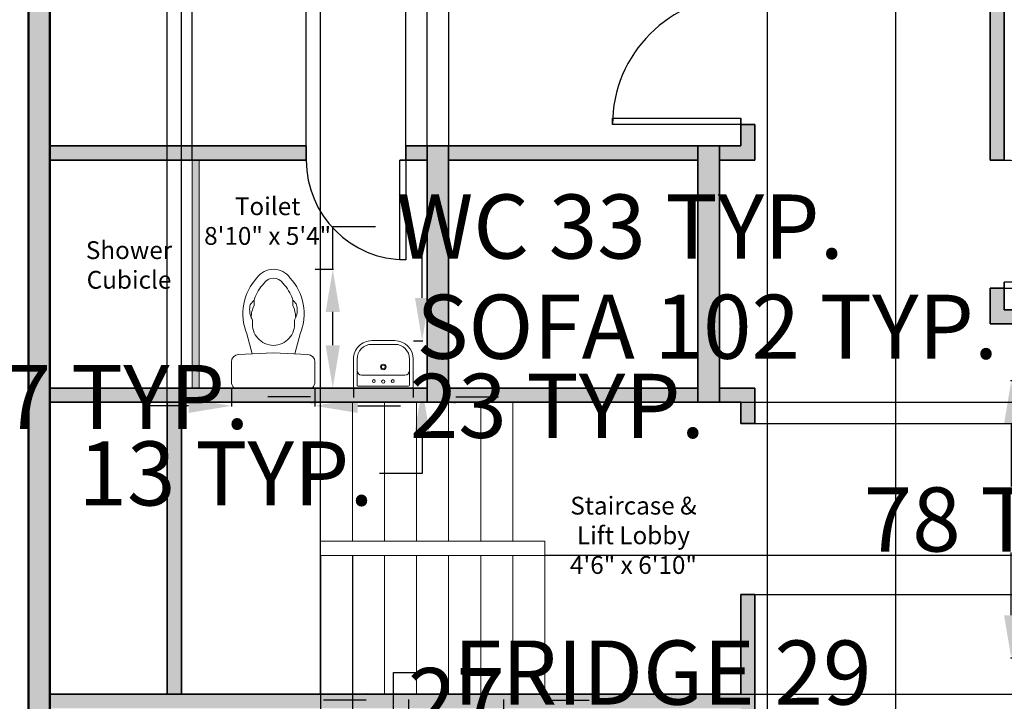
# Model space of a CAD drawing. Units: inches. Extents: x 2 to 695, y -374 to 352.
# Tile 4 of 6: x 144 to 421, y -51 to 141. Entities that reach past the tile are written whole.
import ezdxf

# ---------------------------------------------------------------- set-up
doc = ezdxf.new("R2010")
doc.units = ezdxf.units.IN
for name, color, linetype, lineweight in [('A-ANNO-DIMS', 2, 'Continuous', 18), ('A-ANNO-TEXT', 7, 'Continuous', 18), ('A-AREA-IDEN', 7, 'Continuous', 18), ('A-DOOR', 3, 'Continuous', 25), ('A-FLOR-FIXT', 9, 'Continuous', 18), ('A-FLOR-STRS', 7, 'Continuous', 18), ('A-WALL-PATT', 252, 'Continuous', 13), ('Inner Wall', 5, 'Continuous', 35), ('Outer Wall', 1, 'Continuous', 50)]:
    doc.layers.add(name, color=color, linetype=linetype, lineweight=lineweight)
doc.styles.get("Standard").update_dxf_attribs({"font": 'arial.ttf'})
doc.dimstyles.get("Standard").update_dxf_attribs({"dimtxt": 18, "dimasz": 12, "dimexe": 0.18, "dimexo": 0.0625, "dimgap": 0.09, "dimtad": 0, "dimtih": 1, "dimtoh": 1, "dimdec": 0, "dimzin": 0, "dimdsep": 46, "dimlunit": 3, "dimtxsty": 'Standard', "dimcen": 0.09, "dimadec": 0, "dimazin": 0, "dimtfac": 1, "dimtdec": 0, "dimtofl": 0, "dimtmove": 0, "dimatfit": 3, "dimfxl": 1, "dimtolj": 1, "dimtzin": 0, "dimarcsym": 0})

# ---------------------------------------------------------------- blocks, each defined once
blk = doc.blocks.new('*U2')
for p, q in [((0, 0), (0, -4)), ((36, 0), (36, -4))]:
    blk.add_line(p, q)
blk.add_lwpolyline([(0, 0), (0, 36), (1.75, 36), (1.75, 0)], close=True)
blk.add_arc((0, 0), 36, 0, 90)
blk = doc.blocks.new('A$C1308471B')
at = {"ltscale": 20}
for p, q in [((0, 0.4607), (0, 0.0186)), ((0.0354, 0.4793), (0.1495, 0.4793)), ((0.2013, 0.2397), (0.1923, 0.4384)), ((0.1957, 0.3639), (0.3109, 0.3953)), ((0.5021, 0.3528), (0.4724, 0.3528)), ((0.4982, 0.3575), (0.4822, 0.3709)), ((0.2013, 0.2397), (0.1923, 0.0409)), ((0.1959, 0.1193), (0.3109, 0.0879)), ((0.5021, 0.1304), (0.4724, 0.1304)), ((0.4982, 0.1257), (0.4822, 0.1123)), ((0.0354, 0), (0.1495, 0))]:
    blk.add_line(p, q, dxfattribs=at)
for centre, radius, start, end in [((0.006, 0.4607), 0.006, 136.5269, 180), ((0.0354, 0.4328), 0.0465, 90, 136.5269), ((0.1495, 0.4365), 0.0429, 2.5755, 90), ((0.4248, 0.1104), 0.3068, 47.4135, 111.7924), ((0.3654, 0.2416), 0.1206, 83.3523, 180), ((0.3823, 0.3868), 0.0255, 263.3523, 298.5742), ((0.4494, 0.2636), 0.1148, 79.3968, 118.5742), ((0.405, 0.2159), 0.153, 63.502, 90.4522), ((0.4658, 0.3513), 0.0255, 50, 79.3968), ((0.5146, 0.377), 0.0255, 230, 251.3881), ((0.5021, 0.3273), 0.0255, 70.3751, 90), ((0.4248, 0.1104), 0.2558, 46.612, 70.3751), ((0.5654, 0.2416), 0.065, 0, 57.2974), ((0.5654, 0.2416), 0.116, 0, 54.7115), ((0.3654, 0.2416), 0.1206, 180, 276.6477), ((0.5654, 0.2416), 0.065, 302.7026, 0), ((0.5654, 0.2416), 0.116, 305.2885, 0), ((0.4248, 0.3728), 0.2558, 289.6249, 313.388), ((0.4248, 0.3728), 0.3068, 248.2076, 312.5865), ((0.3823, 0.0964), 0.0255, 61.4258, 96.6477), ((0.4494, 0.2196), 0.1148, 241.4258, 280.6032), ((0.405, 0.2673), 0.153, 269.5478, 296.498), ((0.5146, 0.1062), 0.0255, 108.6119, 130), ((0.5021, 0.1559), 0.0255, 270, 289.6249), ((0.4658, 0.1319), 0.0255, 280.6032, 310), ((0.006, 0.0186), 0.006, 180, 223.4731), ((0.0354, 0.0465), 0.0465, 223.4731, 270), ((0.1495, 0.0429), 0.0429, 270, 357.4245)]:
    blk.add_arc(centre, radius, start, end, dxfattribs=at)
blk = doc.blocks.new('A$C57EA129C')
for p, q in [((0, 0.4428), (0, 0.1782)), ((0.016, 0.4589), (0.5631, 0.4589)), ((0.0356, 0.4321), (0.0356, 0.2896)), ((0.0445, 0.441), (0.5346, 0.441)), ((0.5435, 0.4321), (0.5435, 0.2896)), ((0.5791, 0.4428), (0.5791, 0.1782)), ((0.0356, 0.2896), (0.0356, 0.1782)), ((0.0802, 0.3341), (0.499, 0.3341)), ((0.5435, 0.2896), (0.5435, 0.1782)), ((0.1782, 0.0356), (0.4009, 0.0356)), ((0.1782, 0), (0.4009, 0))]:
    blk.add_line(p, q)
for centre, radius in [((0.1982, 0.392), 0.0143), ((0.2896, 0.3965), 0.0156), ((0.3809, 0.392), 0.0143), ((0.2896, 0.2545), 0.0267), ((0.2896, 0.2545), 0.0178)]:
    blk.add_circle(centre, radius)
for centre, radius, start, end in [((0.016, 0.4428), 0.016, 90, 180), ((0.0445, 0.4321), 0.00891, 90, 180), ((0.5346, 0.4321), 0.00891, 0, 90), ((0.5631, 0.4428), 0.016, 0, 90), ((0.0802, 0.2896), 0.0445, 90, 180), ((0.499, 0.2896), 0.0445, 0, 90), ((0.1782, 0.1782), 0.1782, 180, 270), ((0.1782, 0.1782), 0.1426, 180, 270), ((0.4009, 0.1782), 0.1782, 270, 0), ((0.4009, 0.1782), 0.1426, 270, 0)]:
    blk.add_arc(centre, radius, start, end)
blk = doc.blocks.new('*U3')
for p, q in [((0, 0), (0, -4)), ((28, 0), (28, -4))]:
    blk.add_line(p, q)
blk.add_lwpolyline([(0, 0), (0, 28), (1.75, 28), (1.75, 0)], close=True)
blk.add_arc((0, 0), 28, 0, 90)
blk = doc.blocks.new('*D12')
at = {"layer": 'A-ANNO-DIMS', "color": 0, "lineweight": -2, "transparency": 16777216}
for p, q in [((232.25, 70.53), (232.25, 82.53)), ((232.25, 82.53), (244.25, 82.53)), ((227.31, 70.53), (232.43, 70.53)), ((232.25, 49.18), (232.25, 58.53)), ((227.31, 37.18), (232.43, 37.18))]:
    blk.add_line(p, q, dxfattribs=at)
at = {"layer": 'A-ANNO-DIMS', "color": 0, "transparency": 16777216}
for points in [[(230.25, 58.53), (234.25, 58.53), (232.25, 70.53)], [(230.25, 49.18), (234.25, 49.18), (232.25, 37.18)]]:
    blk.add_solid(points, dxfattribs=at)
at = {"layer": 'Defpoints', "color": 0, "transparency": 16777216}
for p in [(227.24, 70.53), (232.25, 70.53), (227.24, 37.18)]:
    blk.add_point(p, dxfattribs=at)
at = {"layer": 'A-ANNO-DIMS', "color": 0, "transparency": 16777216, "insert": (312.95, 82.53), "char_height": 18, "attachment_point": 5}
blk.add_mtext('\\A1;WC 33 TYP.', dxfattribs=at)
blk = doc.blocks.new('*D13')
at = {"layer": 'A-ANNO-DIMS', "color": 0, "lineweight": -2, "transparency": 16777216}
for p, q in [((203.78, 37.11), (203.78, 31.99)), ((227.24, 37.11), (227.24, 31.99)), ((191.78, 32.17), (179.78, 32.17)), ((239.24, 32.17), (251.24, 32.17))]:
    blk.add_line(p, q, dxfattribs=at)
at = {"layer": 'A-ANNO-DIMS', "color": 0, "transparency": 16777216}
for points in [[(191.78, 34.17), (191.78, 30.17), (203.78, 32.17)], [(239.24, 34.17), (239.24, 30.17), (227.24, 32.17)]]:
    blk.add_solid(points, dxfattribs=at)
at = {"layer": 'Defpoints', "color": 0, "transparency": 16777216}
for p in [(203.78, 37.18), (227.24, 37.18), (227.24, 32.17)]:
    blk.add_point(p, dxfattribs=at)
at = {"layer": 'A-ANNO-DIMS', "color": 0, "transparency": 16777216, "insert": (295.3, 32.17), "char_height": 18, "attachment_point": 5}
blk.add_mtext('\\A1;23 TYP.', dxfattribs=at)
blk = doc.blocks.new('*D14')
at = {"layer": 'A-ANNO-DIMS', "color": 0, "lineweight": -2, "transparency": 16777216}
for p, q in [((238.04, 37.11), (238.04, 34.48)), ((254.82, 37.11), (254.82, 34.48)), ((226.04, 34.66), (214.04, 34.66)), ((266.82, 34.66), (278.82, 34.66))]:
    blk.add_line(p, q, dxfattribs=at)
at = {"layer": 'A-ANNO-DIMS', "color": 0, "transparency": 16777216}
for points in [[(226.04, 36.66), (226.04, 32.66), (238.04, 34.66)], [(266.82, 36.66), (266.82, 32.66), (254.82, 34.66)]]:
    blk.add_solid(points, dxfattribs=at)
at = {"layer": 'Defpoints', "color": 0, "transparency": 16777216}
for p in [(238.04, 37.18), (254.82, 37.18), (238.04, 34.66)]:
    blk.add_point(p, dxfattribs=at)
at = {"layer": 'A-ANNO-DIMS', "color": 0, "transparency": 16777216, "insert": (129.31, 34.66), "char_height": 18, "attachment_point": 5}
blk.add_mtext('\\A1;BASIN 17 TYP.', dxfattribs=at)
blk = doc.blocks.new('*D15')
at = {"layer": 'A-ANNO-DIMS', "color": 0, "lineweight": -2, "transparency": 16777216}
for p, q in [((257.34, 62.47), (257.34, 74.47)), ((254.89, 50.47), (257.52, 50.47)), ((254.89, 37.18), (257.52, 37.18)), ((257.34, 25.18), (257.34, 13.18)), ((257.34, 13.18), (245.34, 13.18))]:
    blk.add_line(p, q, dxfattribs=at)
at = {"layer": 'A-ANNO-DIMS', "color": 0, "transparency": 16777216}
for points in [[(255.34, 62.47), (259.34, 62.47), (257.34, 50.47)], [(255.34, 25.18), (259.34, 25.18), (257.34, 37.18)]]:
    blk.add_solid(points, dxfattribs=at)
at = {"layer": 'Defpoints', "color": 0, "transparency": 16777216}
for p in [(254.82, 50.47), (254.82, 37.18), (257.34, 37.18)]:
    blk.add_point(p, dxfattribs=at)
at = {"layer": 'A-ANNO-DIMS', "color": 0, "transparency": 16777216, "insert": (202.29, 13.18), "char_height": 18, "attachment_point": 5}
blk.add_mtext('\\A1;13 TYP.', dxfattribs=at)
blk = doc.blocks.new('*D18')
at = {"layer": 'A-ANNO-DIMS', "color": 0, "lineweight": -2, "transparency": 16777216}
for p, q in [((437.96, 54.39), (425.96, 54.39)), ((437.96, 39.23), (437.96, 54.57)), ((527.48, 54.39), (449.96, 54.39)), ((539.48, 39.23), (539.48, 54.57))]:
    blk.add_line(p, q, dxfattribs=at)
at = {"layer": 'A-ANNO-DIMS', "color": 0, "transparency": 16777216}
for points in [[(449.96, 56.39), (449.96, 52.39), (437.96, 54.39)], [(527.48, 56.39), (527.48, 52.39), (539.48, 54.39)]]:
    blk.add_solid(points, dxfattribs=at)
at = {"layer": 'Defpoints', "color": 0, "transparency": 16777216}
for p in [(437.96, 54.39), (437.96, 39.17), (539.48, 39.17)]:
    blk.add_point(p, dxfattribs=at)
at = {"layer": 'A-ANNO-DIMS', "color": 0, "transparency": 16777216, "insert": (337.39, 54.39), "char_height": 18, "attachment_point": 5}
blk.add_mtext('\\A1;SOFA 102 TYP.', dxfattribs=at)
blk = doc.blocks.new('*D19')
at = {"layer": 'A-ANNO-DIMS', "color": 0, "lineweight": -2, "transparency": 16777216}
for p, q in [((437.9, 39.17), (422.55, 39.17)), ((422.73, 27.17), (422.73, 9.53)), ((422.73, -26.67), (422.73, -9.03)), ((437.9, -38.67), (422.55, -38.67))]:
    blk.add_line(p, q, dxfattribs=at)
at = {"layer": 'A-ANNO-DIMS', "color": 0, "transparency": 16777216}
for points in [[(420.73, 27.17), (424.73, 27.17), (422.73, 39.17)], [(420.73, -26.67), (424.73, -26.67), (422.73, -38.67)]]:
    blk.add_solid(points, dxfattribs=at)
at = {"layer": 'Defpoints', "color": 0, "transparency": 16777216}
for p in [(437.96, 39.17), (422.73, -38.67), (437.96, -38.67)]:
    blk.add_point(p, dxfattribs=at)
at = {"layer": 'A-ANNO-DIMS', "color": 0, "transparency": 16777216, "insert": (422.73, 0.25), "char_height": 18, "attachment_point": 5}
blk.add_mtext('\\A1;78 TYP.', dxfattribs=at)
blk = doc.blocks.new('*D26')
at = {"layer": 'A-ANNO-DIMS', "color": 0, "lineweight": -2, "transparency": 16777216}
for p, q in [((249.33, -54.75), (249.33, -42.75)), ((249.33, -42.75), (261.33, -42.75)), ((253.55, -54.75), (249.15, -54.75)), ((249.33, -71.32), (249.33, -66.75)), ((253.55, -83.32), (249.15, -83.32))]:
    blk.add_line(p, q, dxfattribs=at)
at = {"layer": 'A-ANNO-DIMS', "color": 0, "transparency": 16777216}
for points in [[(247.33, -66.75), (251.33, -66.75), (249.33, -54.75)], [(247.33, -71.32), (251.33, -71.32), (249.33, -83.32)]]:
    blk.add_solid(points, dxfattribs=at)
at = {"layer": 'Defpoints', "color": 0, "transparency": 16777216}
for p in [(249.33, -54.75), (253.61, -54.75), (253.61, -83.32)]:
    blk.add_point(p, dxfattribs=at)
at = {"layer": 'A-ANNO-DIMS', "color": 0, "transparency": 16777216, "insert": (324.81, -42.75), "char_height": 18, "attachment_point": 5}
blk.add_mtext('\\A1;FRIDGE 29', dxfattribs=at)
blk = doc.blocks.new('*D27')
at = {"layer": 'A-ANNO-DIMS', "color": 0, "lineweight": -2, "transparency": 16777216}
for p, q in [((241.61, -50.46), (229.61, -50.46)), ((253.61, -54.69), (253.61, -50.28)), ((280.28, -54.69), (280.28, -50.28)), ((292.28, -50.46), (304.28, -50.46))]:
    blk.add_line(p, q, dxfattribs=at)
at = {"layer": 'A-ANNO-DIMS', "color": 0, "transparency": 16777216}
for points in [[(241.61, -48.46), (241.61, -52.46), (253.61, -50.46)], [(292.28, -48.46), (292.28, -52.46), (280.28, -50.46)]]:
    blk.add_solid(points, dxfattribs=at)
at = {"layer": 'Defpoints', "color": 0, "transparency": 16777216}
for p in [(280.28, -50.46), (253.61, -54.75), (280.28, -54.75)]:
    blk.add_point(p, dxfattribs=at)
at = {"layer": 'A-ANNO-DIMS', "color": 0, "transparency": 16777216, "insert": (266.94, -50.46), "char_height": 18, "attachment_point": 5}
blk.add_mtext('\\A1;27', dxfattribs=at)
blk = doc.blocks.new('*D29')
at = {"layer": 'A-ANNO-DIMS', "color": 0, "lineweight": -2, "transparency": 16777216}
for p, q in [((420.85, 308.13), (591.88, 308.13)), ((591.7, 296.13), (591.7, -1.56)), ((591.7, -317.82), (591.7, -20.13)), ((217.35, -329.82), (591.88, -329.82))]:
    blk.add_line(p, q, dxfattribs=at)
at = {"layer": 'A-ANNO-DIMS', "color": 0, "transparency": 16777216}
for points in [[(589.7, 296.13), (593.7, 296.13), (591.7, 308.13)], [(589.7, -317.82), (593.7, -317.82), (591.7, -329.82)]]:
    blk.add_solid(points, dxfattribs=at)
at = {"layer": 'Defpoints', "color": 0, "transparency": 16777216}
for p in [(420.79, 308.13), (591.7, 308.13), (217.29, -329.82)]:
    blk.add_point(p, dxfattribs=at)
at = {"layer": 'A-ANNO-DIMS', "color": 0, "transparency": 16777216, "insert": (591.7, -10.85), "char_height": 18, "attachment_point": 5}
blk.add_mtext('\\A1;638', dxfattribs=at)
blk = doc.blocks.new('*D38')
at = {"layer": 'A-ANNO-DIMS', "color": 0, "lineweight": -2, "transparency": 16777216}
for p, q in [((350.85, 27.18), (591.88, 27.18)), ((591.7, 15.18), (591.7, 12.46)), ((591.7, -8.82), (591.7, -6.11)), ((350.85, -20.82), (591.88, -20.82))]:
    blk.add_line(p, q, dxfattribs=at)
at = {"layer": 'A-ANNO-DIMS', "color": 0, "transparency": 16777216}
for points in [[(589.7, 15.18), (593.7, 15.18), (591.7, 27.18)], [(589.7, -8.82), (593.7, -8.82), (591.7, -20.82)]]:
    blk.add_solid(points, dxfattribs=at)
at = {"layer": 'Defpoints', "color": 0, "transparency": 16777216}
for p in [(350.79, 27.18), (350.79, -20.82), (591.7, -20.82)]:
    blk.add_point(p, dxfattribs=at)
at = {"layer": 'A-ANNO-DIMS', "color": 0, "transparency": 16777216, "insert": (591.7, 3.18), "char_height": 18, "attachment_point": 5}
blk.add_mtext('\\A1;48', dxfattribs=at)
blk = doc.blocks.new('*D39')
at = {"layer": 'A-ANNO-DIMS', "color": 0, "lineweight": -2, "transparency": 16777216}
for p, q in [((212.785845, 340.044756), (200.785845, 340.044756)), ((224.785845, 101.237546), (224.785845, 340.224756)), ((252.785845, 101.237546), (252.785845, 340.224756)), ((264.785845, 340.044756), (276.785845, 340.044756))]:
    blk.add_line(p, q, dxfattribs=at)
at = {"layer": 'A-ANNO-DIMS', "color": 0, "transparency": 16777216}
for points in [[(212.785845, 342.044756), (212.785845, 338.044756), (224.785845, 340.044756)], [(264.785845, 342.044756), (264.785845, 338.044756), (252.785845, 340.044756)]]:
    blk.add_solid(points, dxfattribs=at)
at = {"layer": 'Defpoints', "color": 0, "transparency": 16777216}
for p in [(252.785845, 340.044756), (224.785845, 101.175046), (252.785845, 101.175046)]:
    blk.add_point(p, dxfattribs=at)
at = {"layer": 'A-ANNO-DIMS', "color": 0, "transparency": 16777216, "insert": (238.785845, 340.044756), "char_height": 18, "attachment_point": 5}
blk.add_mtext('\\A1;28', dxfattribs=at)
blk = doc.blocks.new('*D40')
at = {"layer": 'A-ANNO-DIMS', "color": 0, "lineweight": -2, "transparency": 16777216}
for p, q in [((140.785845, 340.044756), (128.785845, 340.044756)), ((152.785845, 101.237546), (152.785845, 340.224756)), ((192.785845, 101.237546), (192.785845, 340.224756)), ((204.785845, 340.044756), (216.785845, 340.044756))]:
    blk.add_line(p, q, dxfattribs=at)
at = {"layer": 'A-ANNO-DIMS', "color": 0, "transparency": 16777216}
for points in [[(140.785845, 342.044756), (140.785845, 338.044756), (152.785845, 340.044756)], [(204.785845, 342.044756), (204.785845, 338.044756), (192.785845, 340.044756)]]:
    blk.add_solid(points, dxfattribs=at)
at = {"layer": 'Defpoints', "color": 0, "transparency": 16777216}
for p in [(192.785845, 340.044756), (152.785845, 101.175046), (192.785845, 101.175046)]:
    blk.add_point(p, dxfattribs=at)
at = {"layer": 'A-ANNO-DIMS', "color": 0, "transparency": 16777216, "insert": (172.785845, 340.044756), "char_height": 18, "attachment_point": 5}
blk.add_mtext('\\A1;40', dxfattribs=at)
blk = doc.blocks.new('*D41')
at = {"layer": 'A-ANNO-DIMS', "color": 0, "lineweight": -2, "transparency": 16777216}
for p, q in [((342.285845, 340.044756), (330.285845, 340.044756)), ((354.285845, -164.762454), (354.285845, 340.224756)), ((390.285845, -164.762454), (390.285845, 340.224756)), ((402.285845, 340.044756), (414.285845, 340.044756))]:
    blk.add_line(p, q, dxfattribs=at)
at = {"layer": 'A-ANNO-DIMS', "color": 0, "transparency": 16777216}
for points in [[(342.285845, 342.044756), (342.285845, 338.044756), (354.285845, 340.044756)], [(402.285845, 342.044756), (402.285845, 338.044756), (390.285845, 340.044756)]]:
    blk.add_solid(points, dxfattribs=at)
at = {"layer": 'Defpoints', "color": 0, "transparency": 16777216}
for p in [(390.285845, 340.044756), (354.285845, -164.824954), (390.285845, -164.824954)]:
    blk.add_point(p, dxfattribs=at)
at = {"layer": 'A-ANNO-DIMS', "color": 0, "transparency": 16777216, "insert": (372.285845, 340.044756), "char_height": 18, "attachment_point": 5}
blk.add_mtext('\\A1;36', dxfattribs=at)
blk = doc.blocks.new('*D45')
at = {"layer": 'A-ANNO-DIMS', "color": 0, "lineweight": -2, "transparency": 16777216}
for p, q in [((246.79, 340.04), (234.79, 340.04)), ((258.79, 105.24), (258.79, 340.22)), ((264.79, 105.24), (264.79, 340.22)), ((276.79, 340.04), (288.79, 340.04))]:
    blk.add_line(p, q, dxfattribs=at)
at = {"layer": 'A-ANNO-DIMS', "color": 0, "transparency": 16777216}
for points in [[(246.79, 342.04), (246.79, 338.04), (258.79, 340.04)], [(276.79, 342.04), (276.79, 338.04), (264.79, 340.04)]]:
    blk.add_solid(points, dxfattribs=at)
at = {"layer": 'Defpoints', "color": 0, "transparency": 16777216}
for p in [(264.79, 340.04), (258.79, 105.18), (264.79, 105.18)]:
    blk.add_point(p, dxfattribs=at)
at = {"layer": 'A-ANNO-DIMS', "color": 0, "transparency": 16777216, "insert": (294.82, 340.04), "char_height": 18, "attachment_point": 5}
blk.add_mtext('\\A1;6', dxfattribs=at)
blk = doc.blocks.new('*D46')
at = {"layer": 'A-ANNO-DIMS', "color": 0, "lineweight": -2, "transparency": 16777216}
for p, q in [((140.785845, 340.044756), (128.785845, 340.044756)), ((152.785845, -48.762454), (152.785845, 340.224756)), ((185.785845, -48.762454), (185.785845, 340.224756)), ((197.785845, 340.044756), (209.785845, 340.044756))]:
    blk.add_line(p, q, dxfattribs=at)
at = {"layer": 'A-ANNO-DIMS', "color": 0, "transparency": 16777216}
for points in [[(140.785845, 342.044756), (140.785845, 338.044756), (152.785845, 340.044756)], [(197.785845, 342.044756), (197.785845, 338.044756), (185.785845, 340.044756)]]:
    blk.add_solid(points, dxfattribs=at)
at = {"layer": 'Defpoints', "color": 0, "transparency": 16777216}
for p in [(185.785845, 340.044756), (152.785845, -48.824954), (185.785845, -48.824954)]:
    blk.add_point(p, dxfattribs=at)
at = {"layer": 'A-ANNO-DIMS', "color": 0, "transparency": 16777216, "insert": (169.285845, 340.044756), "char_height": 18, "attachment_point": 5}
blk.add_mtext('\\A1;33', dxfattribs=at)
blk = doc.blocks.new('*D47')
at = {"layer": 'A-ANNO-DIMS', "color": 0, "lineweight": -2, "transparency": 16777216}
for p, q in [((177.785845, 340.044756), (165.785845, 340.044756)), ((189.785845, -48.762454), (189.785845, 340.224756)), ((228.785845, -48.762454), (228.785845, 340.224756)), ((240.785845, 340.044756), (252.785845, 340.044756))]:
    blk.add_line(p, q, dxfattribs=at)
at = {"layer": 'A-ANNO-DIMS', "color": 0, "transparency": 16777216}
for points in [[(177.785845, 342.044756), (177.785845, 338.044756), (189.785845, 340.044756)], [(240.785845, 342.044756), (240.785845, 338.044756), (228.785845, 340.044756)]]:
    blk.add_solid(points, dxfattribs=at)
at = {"layer": 'Defpoints', "color": 0, "transparency": 16777216}
for p in [(228.785845, 340.044756), (189.785845, -48.824954), (228.785845, -48.824954)]:
    blk.add_point(p, dxfattribs=at)
at = {"layer": 'A-ANNO-DIMS', "color": 0, "transparency": 16777216, "insert": (209.285845, 340.044756), "char_height": 18, "attachment_point": 5}
blk.add_mtext('\\A1;39', dxfattribs=at)
blk = doc.blocks.new('*D48')
at = {"layer": 'A-ANNO-DIMS', "color": 0, "lineweight": -2, "transparency": 16777216}
for p, q in [((228.79, -9.89), (228.79, -361.92)), ((237.79, -9.89), (237.79, -361.92)), ((216.79, -361.74), (204.79, -361.74)), ((249.79, -361.74), (261.79, -361.74))]:
    blk.add_line(p, q, dxfattribs=at)
at = {"layer": 'A-ANNO-DIMS', "color": 0, "transparency": 16777216}
for points in [[(216.79, -359.74), (216.79, -363.74), (228.79, -361.74)], [(249.79, -359.74), (249.79, -363.74), (237.79, -361.74)]]:
    blk.add_solid(points, dxfattribs=at)
at = {"layer": 'Defpoints', "color": 0, "transparency": 16777216}
for p in [(228.79, -9.82), (237.79, -9.82), (237.79, -361.74)]:
    blk.add_point(p, dxfattribs=at)
at = {"layer": 'A-ANNO-DIMS', "color": 0, "transparency": 16777216, "insert": (267.79, -361.74), "char_height": 18, "attachment_point": 5}
blk.add_mtext('\\A1;9', dxfattribs=at)
blk = doc.blocks.new('*D49')
at = {"layer": 'A-ANNO-DIMS', "color": 0, "lineweight": -2, "transparency": 16777216}
for p, q in [((591.7, -9.82), (591.7, 2.18)), ((591.7, 2.18), (603.7, 2.18)), ((291.85, -9.82), (591.88, -9.82)), ((591.7, -36.82), (591.7, -21.82)), ((291.85, -48.82), (591.88, -48.82))]:
    blk.add_line(p, q, dxfattribs=at)
at = {"layer": 'A-ANNO-DIMS', "color": 0, "transparency": 16777216}
for points in [[(589.7, -21.82), (593.7, -21.82), (591.7, -9.82)], [(589.7, -36.82), (593.7, -36.82), (591.7, -48.82)]]:
    blk.add_solid(points, dxfattribs=at)
at = {"layer": 'Defpoints', "color": 0, "transparency": 16777216}
for p in [(291.79, -9.82), (591.7, -9.82), (291.79, -48.82)]:
    blk.add_point(p, dxfattribs=at)
at = {"layer": 'A-ANNO-DIMS', "color": 0, "transparency": 16777216, "insert": (616.7, 2.18), "char_height": 18, "attachment_point": 5}
blk.add_mtext('\\A1;39', dxfattribs=at)
blk = doc.blocks.new('*D50')
at = {"layer": 'A-ANNO-DIMS', "color": 0, "lineweight": -2, "transparency": 16777216}
for p, q in [((591.7, 45.18), (591.7, 57.18)), ((346.85, 33.18), (591.88, 33.18)), ((346.85, 27.18), (591.88, 27.18)), ((591.7, 15.18), (591.7, 3.18)), ((591.7, 3.18), (579.7, 3.18))]:
    blk.add_line(p, q, dxfattribs=at)
at = {"layer": 'A-ANNO-DIMS', "color": 0, "transparency": 16777216}
for points in [[(589.7, 45.18), (593.7, 45.18), (591.7, 33.18)], [(589.7, 15.18), (593.7, 15.18), (591.7, 27.18)]]:
    blk.add_solid(points, dxfattribs=at)
at = {"layer": 'Defpoints', "color": 0, "transparency": 16777216}
for p in [(346.79, 33.18), (346.79, 27.18), (591.7, 27.18)]:
    blk.add_point(p, dxfattribs=at)
at = {"layer": 'A-ANNO-DIMS', "color": 0, "transparency": 16777216, "insert": (573.67, 3.18), "char_height": 18, "attachment_point": 5}
blk.add_mtext('\\A1;6', dxfattribs=at)

msp = doc.modelspace()

# ---------------------------------------------------------------- hatches: boundary and pattern name
at = {"layer": 'A-WALL-PATT'}
h = msp.add_hatch(color=256, dxfattribs=at)
h.dxf.hatch_style = 1
h.paths.add_polyline_path([(346.7858, 296.175), (146.7858, 296.175), (146.7858, -329.825), (217.2858, -329.825), (217.2858, -305.825), (559.7858, -305.825), (559.7858, 296.175), (420.7858, 296.175), (420.7858, 290.175), (553.7858, 290.175), (553.7858, -299.825), (213.2858, -299.825), (213.2858, -323.825), (152.7858, -323.825), (152.7858, 290.175), (346.7858, 290.175)])
h.paths.add_polyline_path([(420.7858, 308.1298), (346.7858, 308.1298), (346.7858, 242.175), (228.7858, 242.175), (228.7858, 264.175), (152.7858, 264.175), (152.7858, 260.175), (224.7858, 260.175), (224.7858, 236.175), (350.7858, 236.175), (350.7858, 302.1298), (416.7858, 302.1298), (416.7858, 236.175), (553.7858, 236.175), (553.7858, 242.175), (420.7858, 242.175)])
h = msp.add_hatch(color=256, dxfattribs=at)
h.dxf.hatch_style = 1
h.paths.add_polyline_path([(394.2858, -160.825), (390.2858, -160.825), (390.2858, -164.825), (390.2858, -299.825), (394.2858, -299.825)])
h.paths.add_polyline_path([(217.2858, -235.1253), (213.2858, -235.1253), (213.2858, -299.825), (217.2858, -299.825)])
h.paths.add_polyline_path([(213.2858, -273.825), (152.7858, -273.825), (152.7858, -275.825), (213.2858, -275.825)])
h.paths.add_polyline_path([(354.2858, -160.825), (350.7858, -160.825), (350.7858, -124.825), (346.7858, -124.825), (346.7858, -160.825), (152.7858, -160.825), (152.7858, -164.825), (213.2858, -164.825), (213.2858, -188.8137), (213.2858, -207.1253), (217.2858, -207.1253), (217.2858, -187.1253), (217.2858, -164.825), (354.2858, -164.825)])
h.paths.add_polyline_path([(350.7858, -20.825), (346.7858, -20.825), (346.7858, -48.825), (152.7858, -48.825), (152.7858, -52.825), (249.7858, -52.825), (346.7858, -52.825), (346.7858, -88.825), (350.7858, -88.825)])
h.paths.add_polyline_path([(189.7858, 33.175), (185.7858, 33.175), (185.7858, -48.825), (189.7858, -48.825)])
h.paths.add_polyline_path([(334.7858, 37.175), (264.7858, 37.175), (264.7858, 33.175), (334.7858, 33.175)])
h.paths.add_polyline_path([(258.7858, 37.175), (152.7858, 37.175), (152.7858, 33.175), (258.7858, 33.175)])
h.paths.add_polyline_path([(194.7858, 101.175), (192.7858, 101.175), (192.7858, 37.175), (194.7858, 37.175)])
h.paths.add_polyline_path([(264.7858, 105.175), (258.7858, 105.175), (258.7858, 33.175), (264.7858, 33.175), (264.7858, 37.175)])
h.paths.add_polyline_path([(340.7858, 105.175), (334.7858, 105.175), (334.7858, 33.175), (340.7858, 33.175)])
h.paths.add_polyline_path([(350.7858, 111.175), (346.7858, 111.175), (346.7858, 105.175), (340.7858, 105.175), (340.7858, 101.175), (350.7858, 101.175)])
h.paths.add_polyline_path([(350.7858, 37.175), (340.7858, 37.175), (340.7858, 33.175), (346.7858, 33.175), (346.7858, 27.175), (350.7858, 27.175)])
h.paths.add_polyline_path([(334.7858, 105.175), (264.7858, 105.175), (264.7858, 101.175), (334.7858, 101.175)])
h.paths.add_polyline_path([(258.7858, 105.175), (252.7858, 105.175), (252.7858, 101.175), (258.7858, 101.175)])
h.paths.add_polyline_path([(224.7858, 105.175), (152.7858, 105.175), (152.7858, 101.175), (224.7858, 101.175)])
h.paths.add_polyline_path([(382.7858, 165.1298), (350.7858, 165.1298), (350.7858, 161.1298), (382.7858, 161.1298)])
h.paths.add_polyline_path([(350.7858, 236.175), (346.7858, 236.175), (346.7858, 147.175), (350.7858, 147.175)])
h.paths.add_polyline_path([(420.7858, 202.175), (416.7858, 202.175), (416.7858, 101.175), (420.7858, 101.175)])
h.paths.add_polyline_path([(416.7858, 165.1298), (410.7858, 165.1298), (410.7858, 161.1298), (416.7858, 161.1298)])
h.paths.add_polyline_path([(416.7858, 242.175), (350.7858, 242.175), (350.7858, 240.175), (416.7858, 240.175)])
h.paths.add_polyline_path([(420.7858, 236.175), (416.7858, 236.175), (416.7858, 230.175), (420.7858, 230.175)])
h.paths.add_polyline_path([(553.7858, 59.175), (469.3071, 59.175), (420.7858, 59.175), (420.7858, 65.175), (416.7858, 65.175), (416.7858, 55.175), (553.7858, 55.175)])

# ---------------------------------------------------------------- linework, layer by layer
at = {"layer": 'A-FLOR-FIXT'}
for p, q in [((192.7858, 37.175), (192.7858, 101.175)), ((194.7858, 37.175), (194.7858, 101.175))]:
    msp.add_line(p, q, dxfattribs=at)
at = {"layer": 'A-FLOR-STRS'}
for p, q in [((228.7858, -48.825), (228.7858, 33.175)), ((237.7858, -5.825), (237.7858, 33.175)), ((246.7858, -5.825), (246.7858, 33.175)), ((255.7858, -5.825), (255.7858, 33.175)), ((264.7858, -5.825), (264.7858, 33.175)), ((273.7858, -5.825), (273.7858, 33.175)), ((282.7858, -5.825), (282.7858, 33.175)), ((291.7858, -5.825), (228.7858, -5.825)), ((291.7858, -48.825), (291.7858, -5.825)), ((291.7858, -9.825), (228.7858, -9.825)), ((237.7858, -48.825), (237.7858, -9.825)), ((246.7858, -48.825), (246.7858, -9.825)), ((255.7858, -48.825), (255.7858, -9.825)), ((264.7858, -48.825), (264.7858, -9.825)), ((273.7858, -48.825), (273.7858, -9.825)), ((282.7858, -48.825), (282.7858, -9.825))]:
    msp.add_line(p, q, dxfattribs=at)
at = {"layer": 'Inner Wall'}
for p, q in [((416.7858, 101.175), (416.7858, 202.175)), ((420.7858, 101.175), (420.7858, 202.175)), ((346.7858, 105.175), (346.7858, 112.925)), ((350.7858, 111.175), (346.7858, 111.175)), ((350.7858, 111.175), (350.7858, 101.175)), ((224.7858, 105.175), (152.7858, 105.175)), ((224.7858, 101.175), (224.7858, 105.175)), ((346.7858, 105.175), (252.7858, 105.175)), ((252.7858, 105.175), (252.7858, 101.175)), ((258.7858, 33.175), (258.7858, 105.175)), ((264.7858, 33.175), (264.7858, 105.175)), ((334.7858, 33.175), (334.7858, 105.175)), ((340.7858, 33.175), (340.7858, 105.175)), ((224.7858, 101.175), (152.7858, 101.175)), ((258.7858, 101.175), (251.0358, 101.175)), ((334.7858, 101.175), (264.7858, 101.175)), ((350.7858, 101.175), (340.7858, 101.175)), ((416.7858, 101.175), (420.7858, 101.175)), ((420.7858, 59.175), (420.7858, 66.925)), ((416.7858, 55.175), (416.7858, 65.175)), ((416.7858, 65.175), (420.7858, 65.175)), ((420.7858, 59.175), (553.7858, 59.175)), ((416.7858, 55.175), (553.7858, 55.175)), ((258.7858, 37.175), (152.7858, 37.175)), ((334.7858, 37.175), (264.7858, 37.175)), ((350.7858, 37.175), (340.7858, 37.175)), ((350.7858, 27.175), (350.7858, 37.175)), ((346.7858, 33.175), (152.7858, 33.175)), ((185.7858, -48.825), (185.7858, 33.175)), ((189.7858, -48.825), (189.7858, 33.175)), ((346.7858, 27.175), (346.7858, 33.175)), ((350.7858, 27.175), (346.7858, 27.175)), ((346.7858, -48.825), (346.7858, -20.825)), ((350.7858, -20.825), (346.7858, -20.825)), ((350.7858, -88.825), (350.7858, -20.825)), ((346.7858, -48.825), (152.7858, -48.825))]:
    msp.add_line(p, q, dxfattribs=at)
at = {"layer": 'Outer Wall'}
for p, q in [((146.7858, -329.825), (146.7858, 296.175)), ((152.7858, -323.825), (152.7858, 290.175))]:
    msp.add_line(p, q, dxfattribs=at)

# ---------------------------------------------------------------- block references
at = {"layer": 'A-DOOR'}
for name, p, rotation in [('*U2', (346.7858, 111.175), 89.99999999999999), ('*U3', (252.7858, 101.175), 180.0000000000001)]:
    msp.add_blockref(name, p, dxfattribs=dict(at, rotation=rotation))
at = {"layer": 'A-DOOR', "xscale": -1, "rotation": 270}
msp.add_blockref('*U2', (420.7858, 65.175), dxfattribs=at)
at = {"layer": 'A-FLOR-FIXT'}
for name, p, xscale, yscale, zscale, rotation in [('A$C1308471B', (203.7764, 37.175), -48.95497407897215, 48.95497407897215, 48.95497407897215, 270.0000000000001), ('A$C57EA129C', (254.823, 50.4745), 28.98333223671166, 28.98333223671166, 28.98333223671166, 180)]:
    msp.add_blockref(name, p, dxfattribs=dict(at, xscale=xscale, yscale=yscale, zscale=zscale, rotation=rotation))

# ---------------------------------------------------------------- texts
at = {"layer": 'A-ANNO-TEXT', "insert": (199.5986, 78.4024), "char_height": 5, "attachment_point": 3}
msp.add_mtext_dynamic_manual_height_columns('\\pxqc;{\\fTimes New Roman|b0|i0|c0|p18;Shower\\PCubicle}', width=49.101878, gutter_width=12.5, heights=[0], dxfattribs=at)
at = {"layer": 'A-AREA-IDEN', "char_height": 5, "attachment_point": 3}
for s, insert in [('\\pxqc;{\\fTimes New Roman|b0|i0|c0|p18;Toilet\\P8\'10" x 5\'4"}', (238.5139, 90.7292)), ('\\pxqc;{\\fTimes New Roman|b0|i0|c0|p18;Staircase &\\PLift Lobby\\P4\'6" x 6\'10"}', (341.2193, 6.6318))]:
    msp.add_mtext_dynamic_manual_height_columns(s, width=49.101878, gutter_width=12.5, heights=[0], dxfattribs=dict(at, insert=insert))

# ---------------------------------------------------------------- dimensions: what is measured, and where the dimension line sits
at = {"layer": 'A-ANNO-DIMS'}
for base, p1, p2, picture, middle in [((192.7858, 340.0448), (152.7858, 101.175), (192.7858, 101.175), '*D40', (172.7858, 340.0448)), ((185.7858, 340.0448), (152.7858, -48.825), (185.7858, -48.825), '*D46', (169.2858, 340.0448)), ((228.7858, 340.0448), (189.7858, -48.825), (228.7858, -48.825), '*D47', (209.2858, 340.0448)), ((252.7858, 340.0448), (224.7858, 101.175), (252.7858, 101.175), '*D39', (238.7858, 340.0448)), ((264.7858, 340.0448), (258.7858, 105.175), (264.7858, 105.175), '*D45', (294.8185, 340.0448)), ((390.2858, 340.0448), (354.2858, -164.825), (390.2858, -164.825), '*D41', (372.2858, 340.0448)), ((237.7858, -361.74), (228.7858, -9.825), (237.7858, -9.825), '*D48', (267.794, -361.74)), ((280.2766, -50.4633), (253.6113, -54.7488), (280.2766, -54.7488), '*D27', (266.944, -50.4633))]:
    dim = msp.add_linear_dim(base=base, p1=p1, p2=p2, dimstyle='Standard', override={"dimdec": 0, "dimlfac": 1, "dimrnd": 0, "dimzin": 0, "dimdsep": 46, "dimlunit": 2}, dxfattribs=at)
    dim.commit()
    dim.dimension.update_dxf_attribs({"geometry": picture, "text_midpoint": middle})
for base, p1, p2, picture, middle in [((591.7008, 308.1298), (217.2858, -329.825), (420.7858, 308.1298), '*D29', (591.7008, -10.8476)), ((591.7008, 27.175), (346.7858, 33.175), (346.7858, 27.175), '*D50', (573.6681, 3.175)), ((591.7008, -20.825), (350.7858, 27.175), (350.7858, -20.825), '*D38', (591.7008, 3.175)), ((591.7008, -9.825), (291.7858, -48.825), (291.7858, -9.825), '*D49', (616.6953, 2.175))]:
    dim = msp.add_linear_dim(base=base, p1=p1, p2=p2, angle=90, dimstyle='Standard', override={"dimdec": 0, "dimlfac": 1, "dimrnd": 0, "dimzin": 0, "dimdsep": 46, "dimlunit": 2}, dxfattribs=at)
    dim.commit()
    dim.dimension.update_dxf_attribs({"geometry": picture, "text_midpoint": middle})
for base, p1, p2, angle, text, picture, middle in [((232.2464, 70.5318), (227.2429, 37.175), (227.2429, 70.5318), 90, 'WC <> TYP.', '*D12', (312.9537, 82.5318)), ((437.9621, 54.3935), (539.4825, 39.1654), (437.9621, 39.1654), 180, 'SOFA <> TYP.', '*D18', (337.3885, 54.3935)), ((238.0373, 34.6572), (254.823, 37.175), (238.0373, 37.175), 180, 'BASIN <> TYP.', '*D14', (129.3129, 34.6572)), ((257.3408, 37.175), (254.823, 50.4745), (254.823, 37.175), 270, '<> TYP.', '*D15', (202.289, 13.175)), ((227.2429, 32.1715), (203.7764, 37.175), (227.2429, 37.175), 0, '<> TYP.', '*D13', (295.2954, 32.1715)), ((422.7341, -38.6669), (437.9621, 39.1654), (437.9621, -38.6669), 270, '<> TYP.', '*D19', (422.7341, 0.2493)), ((249.3258, -54.7488), (253.6113, -83.3188), (253.6113, -54.7488), 90, 'FRIDGE <>', '*D26', (324.8087, -42.7488))]:
    dim = msp.add_linear_dim(base=base, p1=p1, p2=p2, angle=angle, text=text, dimstyle='Standard', override={"dimdec": 0, "dimlfac": 1, "dimrnd": 0, "dimzin": 0, "dimdsep": 46, "dimlunit": 2}, dxfattribs=at)
    dim.commit()
    dim.dimension.update_dxf_attribs({"geometry": picture, "text_midpoint": middle})

doc.saveas('drawing.dxf')
